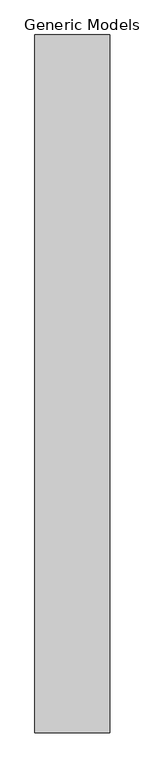
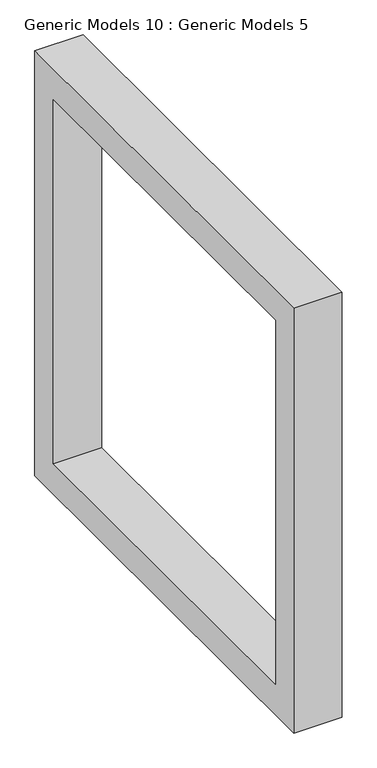
"""IFC4 building model written with IfcOpenShell, lengths in millimetres: proxy geometry, Generic Models 10 : Generic Models 5."""

from ifc_helpers import new_model, si_unit, frame, origin, place, context, project, spatial, polyline, outline, extrude, source, transform, mapped, element, save


def generic_models_10_generic_models_5_40bb8100(model_context):
    return source(origin(), model_context, "Body", "SweptSolid", [
        extrude(outline(polyline([(-6413.4620333, 11769.6), (-6413.4620333, 10347.2), (-7835.8620333, 10347.2), (-7835.8620333, 11769.6), (-6413.4620333, 11769.6)]), holes=[polyline([(-6515.0620333, 11668.0), (-7734.2620333, 11668.0), (-7734.2620333, 10448.8), (-6515.0620333, 10448.8), (-6515.0620333, 11668.0)])]), frame((9218.6824202, 0.0, 0.0), z_axis=(1.0, 0.0, 0.0), x_axis=(0.0, 1.0, 0.0)), (0.0, 0.0, 1.0), 152.4),
    ])


if __name__ == "__main__":
    model = new_model("IFC4")
    model_context = context("Model", 3, world=origin())
    ifc_project = project(units=[si_unit("LENGTHUNIT", "METRE", prefix="MILLI")], contexts=[model_context])
    site = spatial("IfcSite", under=ifc_project)
    building = spatial("IfcBuilding", under=site)
    placement = place(None, origin())
    generic_models_10_generic_models_5_shape = generic_models_10_generic_models_5_40bb8100(model_context)
    element("IfcBuildingElementProxy", 1, Name="Generic Models 10 : Generic Models 5", ObjectType="Generic Models 10 : Generic Models 5", at=placement, inside=building, context=model_context, shape_type="MappedRepresentation", body=[
        mapped(generic_models_10_generic_models_5_shape, transform((0.0, 0.0, 0.0), x_axis=(1.0, 0.0, 0.0), y_axis=(0.0, 1.0, 0.0), z_axis=(0.0, 0.0, 1.0))),
    ])
    save(model, "model.ifc")

# Revit data of these elements
# Element 1 (IfcBuildingElementProxy, "Generic Models 10 : Generic Models 5")
#   Materials on its faces: "black accent wall"
# Materials
#   "black accent wall": class "Generic", colour RGB 120 120 120, transparency 0, Cost = 0
